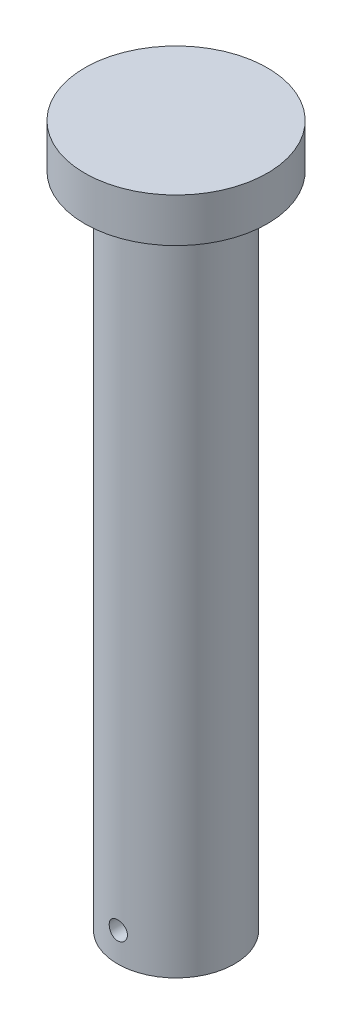
ISO-10303-21;
HEADER;
FILE_DESCRIPTION(('STEP AP214'),'2;1');
FILE_NAME('part.step','',(''),(''),'','','');
FILE_SCHEMA(('AUTOMOTIVE_DESIGN { 1 0 10303 214 1 1 1 1 }'));
ENDSEC;
DATA;
#1=APPLICATION_CONTEXT('core data for automotive mechanical design processes');
#2=APPLICATION_PROTOCOL_DEFINITION('international standard','automotive_design',2000,#1);
#3=PRODUCT_CONTEXT('',#1,'mechanical');
#4=PRODUCT('Part','Part','',(#3));
#5=PRODUCT_RELATED_PRODUCT_CATEGORY('part','',(#4));
#6=PRODUCT_DEFINITION_FORMATION('','',#4);
#7=PRODUCT_DEFINITION_CONTEXT('part definition',#1,'design');
#8=PRODUCT_DEFINITION('design','',#6,#7);
#9=PRODUCT_DEFINITION_SHAPE('','',#8);
#10=(LENGTH_UNIT() NAMED_UNIT(*) SI_UNIT(.MILLI.,.METRE.));
#11=(NAMED_UNIT(*) PLANE_ANGLE_UNIT() SI_UNIT($,.RADIAN.));
#12=(NAMED_UNIT(*) SI_UNIT($,.STERADIAN.) SOLID_ANGLE_UNIT());
#13=UNCERTAINTY_MEASURE_WITH_UNIT(LENGTH_MEASURE(1.E-05),#10,'distance_accuracy_value','');
#14=(GEOMETRIC_REPRESENTATION_CONTEXT(3) GLOBAL_UNCERTAINTY_ASSIGNED_CONTEXT((#13)) GLOBAL_UNIT_ASSIGNED_CONTEXT((#10,
#11,#12)) REPRESENTATION_CONTEXT('',''));
#15=CARTESIAN_POINT('',(0.,0.,0.));
#16=DIRECTION('',(0.,0.,1.));
#17=DIRECTION('',(1.,0.,0.));
#18=AXIS2_PLACEMENT_3D('',#15,#16,#17);
#19=CARTESIAN_POINT('',(0.,12.,0.));
#20=DIRECTION('',(0.,-1.,0.));
#21=DIRECTION('',(0.,0.,-1.));
#22=AXIS2_PLACEMENT_3D('',#19,#20,#21);
#23=CYLINDRICAL_SURFACE('',#22,25.);
#24=CARTESIAN_POINT('',(0.,12.,0.));
#25=DIRECTION('',(0.,1.,0.));
#26=DIRECTION('',(0.,0.,1.));
#27=AXIS2_PLACEMENT_3D('',#24,#25,#26);
#28=CIRCLE('',#27,25.);
#29=CARTESIAN_POINT('',(0.,12.,25.));
#30=VERTEX_POINT('',#29);
#31=EDGE_CURVE('E51',#30,#30,#28,.T.);
#32=ORIENTED_EDGE('',*,*,#31,.F.);
#33=EDGE_LOOP('',(#32));
#34=FACE_BOUND('',#33,.T.);
#35=CARTESIAN_POINT('',(0.,0.,0.));
#36=DIRECTION('',(0.,1.,0.));
#37=DIRECTION('',(0.,0.,1.));
#38=AXIS2_PLACEMENT_3D('',#35,#36,#37);
#39=CIRCLE('',#38,25.);
#40=CARTESIAN_POINT('',(0.,0.,25.));
#41=VERTEX_POINT('',#40);
#42=EDGE_CURVE('E57',#41,#41,#39,.T.);
#43=ORIENTED_EDGE('',*,*,#42,.T.);
#44=EDGE_LOOP('',(#43));
#45=FACE_BOUND('',#44,.T.);
#46=ADVANCED_FACE('F39',(#34,#45),#23,.T.);
#47=CARTESIAN_POINT('',(0.,12.,0.));
#48=DIRECTION('',(0.,1.,0.));
#49=DIRECTION('',(0.,0.,1.));
#50=AXIS2_PLACEMENT_3D('',#47,#48,#49);
#51=PLANE('',#50);
#52=ORIENTED_EDGE('',*,*,#31,.T.);
#53=EDGE_LOOP('',(#52));
#54=FACE_BOUND('',#53,.T.);
#55=ADVANCED_FACE('F87',(#54),#51,.T.);
#56=CARTESIAN_POINT('',(0.,0.,0.));
#57=DIRECTION('',(0.,1.,0.));
#58=DIRECTION('',(0.,0.,1.));
#59=AXIS2_PLACEMENT_3D('',#56,#57,#58);
#60=PLANE('',#59);
#61=CARTESIAN_POINT('',(0.,0.,0.));
#62=DIRECTION('',(0.,-1.,0.));
#63=DIRECTION('',(0.,0.,-1.));
#64=AXIS2_PLACEMENT_3D('',#61,#62,#63);
#65=CIRCLE('',#64,16.);
#66=CARTESIAN_POINT('',(0.,0.,-16.));
#67=VERTEX_POINT('',#66);
#68=EDGE_CURVE('E10',#67,#67,#65,.T.);
#69=ORIENTED_EDGE('',*,*,#68,.F.);
#70=EDGE_LOOP('',(#69));
#71=FACE_BOUND('',#70,.T.);
#72=ORIENTED_EDGE('',*,*,#42,.F.);
#73=EDGE_LOOP('',(#72));
#74=FACE_BOUND('',#73,.T.);
#75=ADVANCED_FACE('F82',(#71,#74),#60,.F.);
#76=CARTESIAN_POINT('',(0.,-180.,0.));
#77=DIRECTION('',(0.,1.,0.));
#78=DIRECTION('',(0.,0.,1.));
#79=AXIS2_PLACEMENT_3D('',#76,#77,#78);
#80=CYLINDRICAL_SURFACE('',#79,16.);
#81=CARTESIAN_POINT('',(0.,-174.5,16.));
#82=CARTESIAN_POINT('',(-0.139515097271032,-174.499994301728,15.9999977019448));
#83=CARTESIAN_POINT('',(-0.279109404865702,-174.488281886226,15.9981561248574));
#84=CARTESIAN_POINT('',(-0.554391314978101,-174.441756308723,15.9909869809759));
#85=CARTESIAN_POINT('',(-0.690075061323318,-174.406921107496,15.9856560884472));
#86=CARTESIAN_POINT('',(-0.953512538047406,-174.315220337193,15.9721069716578));
#87=CARTESIAN_POINT('',(-1.08127235228991,-174.258371918638,15.9638909956317));
#88=CARTESIAN_POINT('',(-1.3254212510446,-174.124301454858,15.9454779403815));
#89=CARTESIAN_POINT('',(-1.44181181036831,-174.047082056964,15.9352811186255));
#90=CARTESIAN_POINT('',(-1.66091991165162,-173.873766951646,15.9139426841436));
#91=CARTESIAN_POINT('',(-1.76352747914264,-173.77753300511,15.9027945139234));
#92=CARTESIAN_POINT('',(-1.95120768822823,-173.569218051731,15.8808607613029));
#93=CARTESIAN_POINT('',(-2.03627928654192,-173.4571361027,15.8700752005075));
#94=CARTESIAN_POINT('',(-2.18690544328884,-173.219561728656,15.8500242812744));
#95=CARTESIAN_POINT('',(-2.25235273557992,-173.094000517638,15.840767397861));
#96=CARTESIAN_POINT('',(-2.36118681597066,-172.833498589142,15.8249120174236));
#97=CARTESIAN_POINT('',(-2.40457491010064,-172.698558427489,15.8183133630222));
#98=CARTESIAN_POINT('',(-2.46771559322167,-172.424289098856,15.8085863451104));
#99=CARTESIAN_POINT('',(-2.48765705487496,-172.285004414181,15.8054302653236));
#100=CARTESIAN_POINT('',(-2.50392369757622,-172.005032811107,15.8028617107177));
#101=CARTESIAN_POINT('',(-2.50025034860466,-171.864345980534,15.8034490028802));
#102=CARTESIAN_POINT('',(-2.4695458080889,-171.586902968147,15.8082755045521));
#103=CARTESIAN_POINT('',(-2.44272562959694,-171.450122776647,15.8124817218495));
#104=CARTESIAN_POINT('',(-2.36681937833752,-171.183027993641,15.8240205634547));
#105=CARTESIAN_POINT('',(-2.31773262684132,-171.052713599359,15.8313532830641));
#106=CARTESIAN_POINT('',(-2.19846916949384,-170.801611287323,15.8483550685462));
#107=CARTESIAN_POINT('',(-2.12820372315549,-170.680866208227,15.8580339308724));
#108=CARTESIAN_POINT('',(-1.96864058146637,-170.452800464314,15.878630461501));
#109=CARTESIAN_POINT('',(-1.87934153253016,-170.345480755113,15.8895482178821));
#110=CARTESIAN_POINT('',(-1.68309088822332,-170.146089753367,15.911537862489));
#111=CARTESIAN_POINT('',(-1.57595800560537,-170.054196841731,15.9226101363559));
#112=CARTESIAN_POINT('',(-1.34769694737934,-169.88966685436,15.9435512534783));
#113=CARTESIAN_POINT('',(-1.22656870068131,-169.817029876443,15.9534200906202));
#114=CARTESIAN_POINT('',(-0.97359592705649,-169.693061926578,15.9708539902704));
#115=CARTESIAN_POINT('',(-0.841744186240456,-169.641745441467,15.9784174854193));
#116=CARTESIAN_POINT('',(-0.571149534696756,-169.562034032553,15.9903756000068));
#117=CARTESIAN_POINT('',(-0.4324071306872,-169.533637425934,15.9947704520898));
#118=CARTESIAN_POINT('',(-0.153508336763736,-169.50081072355,15.9998651172728));
#119=CARTESIAN_POINT('',(-0.0133814615086998,-169.496135521024,16.0006027179286));
#120=CARTESIAN_POINT('',(0.265654546411646,-169.510232705336,15.9984028649127));
#121=CARTESIAN_POINT('',(0.404563719925158,-169.529004302589,15.9954655349964));
#122=CARTESIAN_POINT('',(0.676473446265712,-169.58925838768,15.9862692369322));
#123=CARTESIAN_POINT('',(0.809501262056055,-169.630620758268,15.9800278421539));
#124=CARTESIAN_POINT('',(1.06673406785664,-169.734755094399,15.9649207568356));
#125=CARTESIAN_POINT('',(1.19093861303941,-169.797528138443,15.9560549341007));
#126=CARTESIAN_POINT('',(1.42807220225041,-169.943271991127,15.9365897274094));
#127=CARTESIAN_POINT('',(1.54090512378373,-170.02639742009,15.9259772866342));
#128=CARTESIAN_POINT('',(1.75110696507807,-170.210272085908,15.9042388046444));
#129=CARTESIAN_POINT('',(1.84847490447018,-170.311022439205,15.8931127309268));
#130=CARTESIAN_POINT('',(2.02588080776692,-170.528381197217,15.8714802753665));
#131=CARTESIAN_POINT('',(2.10575398584129,-170.645124847122,15.860980411908));
#132=CARTESIAN_POINT('',(2.24475567726643,-170.890516073661,15.8419069280583));
#133=CARTESIAN_POINT('',(2.30388478778106,-171.019163307489,15.83333325222));
#134=CARTESIAN_POINT('',(2.39946771944995,-171.284229640714,15.8191307135236));
#135=CARTESIAN_POINT('',(2.43600654947913,-171.420617468766,15.8134908234896));
#136=CARTESIAN_POINT('',(2.48564122040535,-171.697689143664,15.8057657028079));
#137=CARTESIAN_POINT('',(2.49873883084997,-171.838372665419,15.8036802038444));
#138=CARTESIAN_POINT('',(2.50107452690756,-172.118398715907,15.8033105804488));
#139=CARTESIAN_POINT('',(2.49057180548425,-172.257739096933,15.804985160429));
#140=CARTESIAN_POINT('',(2.44656223255901,-172.532645297144,15.8118569894183));
#141=CARTESIAN_POINT('',(2.41305543086961,-172.668211124502,15.8170542307995));
#142=CARTESIAN_POINT('',(2.32408329891852,-172.93163782664,15.8303708885491));
#143=CARTESIAN_POINT('',(2.26863761738581,-173.059505478258,15.8384876895341));
#144=CARTESIAN_POINT('',(2.13738768546418,-173.304165613676,15.856731840474));
#145=CARTESIAN_POINT('',(2.06158262820886,-173.420957658288,15.8668592701083));
#146=CARTESIAN_POINT('',(1.89083008139079,-173.641465544127,15.8881156809226));
#147=CARTESIAN_POINT('',(1.79569107094767,-173.745032196614,15.8992540116029));
#148=CARTESIAN_POINT('',(1.58937594638203,-173.934821236387,15.9212004364073));
#149=CARTESIAN_POINT('',(1.47819612078432,-174.021039598592,15.9320084534012));
#150=CARTESIAN_POINT('',(1.24216685884341,-174.174151223032,15.952151024567));
#151=CARTESIAN_POINT('',(1.11723937214237,-174.24092537276,15.9614763443027));
#152=CARTESIAN_POINT('',(0.857851882357781,-174.352440996193,15.9775125983888));
#153=CARTESIAN_POINT('',(0.723401776581768,-174.397204972558,15.9842262014212));
#154=CARTESIAN_POINT('',(0.490314239911604,-174.453433021091,15.9927744586488));
#155=CARTESIAN_POINT('',(0.393105575651631,-174.470868490629,15.9954699162612));
#156=CARTESIAN_POINT('',(0.197277797850584,-174.494153913379,15.9990834869762));
#157=CARTESIAN_POINT('',(0.0986587041691198,-174.500004029557,16.0000016250796));
#158=CARTESIAN_POINT('',(0.,-174.5,16.));
#159=B_SPLINE_CURVE_WITH_KNOTS('',3,(#81,#82,#83,#84,#85,#86,#87,#88,#89,#90,#91,#92,#93,#94,
#95,#96,#97,#98,#99,#100,#101,#102,#103,#104,#105,#106,#107,#108,#109,#110,#111,#112,#113,#114,
#115,#116,#117,#118,#119,#120,#121,#122,#123,#124,#125,#126,#127,#128,#129,#130,#131,#132,#133,
#134,#135,#136,#137,#138,#139,#140,#141,#142,#143,#144,#145,#146,#147,#148,#149,#150,#151,#152,
#153,#154,#155,#156,#157,#158),.UNSPECIFIED.,.T.,.F.,(4,2,2,2,2,2,2,2,2,2,2,2,2,2,2,2,2,2,2,2,2,
2,2,2,2,2,2,2,2,2,2,2,2,2,2,2,2,2,4),(0.,0.418184740477489,0.836768642528017,1.25502707944104,
1.6732311879203,2.09459568152198,2.51598523645421,2.9396377860576,3.36326525009242,
3.78345631134993,4.20362121670544,4.61999576022579,5.0363829965105,5.45453977402348,
5.87272629892068,6.29545732334371,6.71819049513828,7.14121043754565,7.56419931829866,
7.98280854005915,8.40140366528357,8.81779444756568,9.23420620742031,9.65388541469672,
10.0735912160142,10.497094802496,10.9205861964898,11.3424741039513,11.764330162293,
12.1815758159869,12.598820566189,13.0156924696662,13.4325808967135,13.8538201231554,
14.275156971423,14.6990230419984,15.1224548565628,15.4181801635154,15.7139013105871),.UNSPECIFIED.);
#160=CARTESIAN_POINT('',(0.,-174.5,16.));
#161=VERTEX_POINT('',#160);
#162=EDGE_CURVE('E45',#161,#161,#159,.T.);
#163=ORIENTED_EDGE('',*,*,#162,.T.);
#164=EDGE_LOOP('',(#163));
#165=FACE_BOUND('',#164,.T.);
#166=CARTESIAN_POINT('',(2.5,-172.,-15.8034806292791));
#167=CARTESIAN_POINT('',(2.49999429179104,-171.860496621659,-15.8034830346332));
#168=CARTESIAN_POINT('',(2.48828377742084,-171.720914002315,-15.8053478026579));
#169=CARTESIAN_POINT('',(2.44176643645043,-171.445656370997,-15.8125997089633));
#170=CARTESIAN_POINT('',(2.40693752801736,-171.309985224521,-15.8179902148259));
#171=CARTESIAN_POINT('',(2.31525516047132,-171.046574410356,-15.8316684916183));
#172=CARTESIAN_POINT('',(2.25841914921921,-170.918828552129,-15.8399539668268));
#173=CARTESIAN_POINT('',(2.12437791816389,-170.674703109158,-15.8584858981599));
#174=CARTESIAN_POINT('',(2.04717531605121,-170.55832206634,-15.8687321022282));
#175=CARTESIAN_POINT('',(1.8738773011091,-170.339203514849,-15.8901303851737));
#176=CARTESIAN_POINT('',(1.77763988617498,-170.2365789256,-15.9012888784461));
#177=CARTESIAN_POINT('',(1.5693108098767,-170.04886577957,-15.9231973082666));
#178=CARTESIAN_POINT('',(1.45721825316847,-169.963778213776,-15.9339472216984));
#179=CARTESIAN_POINT('',(1.2196342918576,-169.813135122959,-15.9538946715316));
#180=CARTESIAN_POINT('',(1.09407592635728,-169.747683996026,-15.9630838016344));
#181=CARTESIAN_POINT('',(0.833580171794749,-169.638842045275,-15.978803149105));
#182=CARTESIAN_POINT('',(0.698643320136801,-169.595449958617,-15.9853335186778));
#183=CARTESIAN_POINT('',(0.424385325448801,-169.532301281044,-15.9949542857973));
#184=CARTESIAN_POINT('',(0.285108760160741,-169.512355350932,-15.9980722260505));
#185=CARTESIAN_POINT('',(0.0051531435506613,-169.496076956697,-16.0006113098095));
#186=CARTESIAN_POINT('',(-0.135525822989196,-169.499743073648,-16.0000326754547));
#187=CARTESIAN_POINT('',(-0.413000089722162,-169.530435926278,-15.9952657389868));
#188=CARTESIAN_POINT('',(-0.549818542575187,-169.55725893884,-15.9911089169598));
#189=CARTESIAN_POINT('',(-0.816988375343502,-169.633184028623,-15.9796877395528));
#190=CARTESIAN_POINT('',(-0.947339577352183,-169.682286718354,-15.9724232987387));
#191=CARTESIAN_POINT('',(-1.19848742679248,-169.80158365586,-15.9555491842028));
#192=CARTESIAN_POINT('',(-1.31924299071838,-169.871863005428,-15.9459300777042));
#193=CARTESIAN_POINT('',(-1.54732385653215,-170.031456080629,-15.9254174702046));
#194=CARTESIAN_POINT('',(-1.65464819959325,-170.120771163955,-15.9145238783282));
#195=CARTESIAN_POINT('',(-1.85402198520022,-170.317033487073,-15.8925387825556));
#196=CARTESIAN_POINT('',(-1.94589625613073,-170.424158666395,-15.8814464071021));
#197=CARTESIAN_POINT('',(-2.11039226047484,-170.652397564682,-15.8604269384475));
#198=CARTESIAN_POINT('',(-2.18301385538335,-170.773511384274,-15.8504998536298));
#199=CARTESIAN_POINT('',(-2.30697060635686,-171.026479628106,-15.8329349281613));
#200=CARTESIAN_POINT('',(-2.35828663884161,-171.158343575073,-15.8252991458489));
#201=CARTESIAN_POINT('',(-2.43799343127668,-171.428964848705,-15.8132168990948));
#202=CARTESIAN_POINT('',(-2.46638595195258,-171.56772164507,-15.8087701897074));
#203=CARTESIAN_POINT('',(-2.49919719237856,-171.846628103275,-15.8036163696886));
#204=CARTESIAN_POINT('',(-2.50386473411271,-171.986747800195,-15.80287044806));
#205=CARTESIAN_POINT('',(-2.48975479033184,-172.265767635298,-15.8050994977182));
#206=CARTESIAN_POINT('',(-2.47097809654328,-172.404667814506,-15.8080743433524));
#207=CARTESIAN_POINT('',(-2.41072412555895,-172.676527807466,-15.8173740105186));
#208=CARTESIAN_POINT('',(-2.36937178781978,-172.80951599864,-15.8236803883335));
#209=CARTESIAN_POINT('',(-2.26527072241931,-173.066673971104,-15.8389172439685));
#210=CARTESIAN_POINT('',(-2.20252085602949,-173.190843282649,-15.8478478614411));
#211=CARTESIAN_POINT('',(-2.05681199170293,-173.427951281649,-15.8674179220711));
#212=CARTESIAN_POINT('',(-1.9736925109347,-173.5407902289,-15.8780706945976));
#213=CARTESIAN_POINT('',(-1.78982593995281,-173.751006980848,-15.8998450469621));
#214=CARTESIAN_POINT('',(-1.6890777652142,-173.848383833607,-15.9109666556111));
#215=CARTESIAN_POINT('',(-1.47171546765808,-174.025811270635,-15.9325473887455));
#216=CARTESIAN_POINT('',(-1.35496564158983,-174.10569657643,-15.9429995842164));
#217=CARTESIAN_POINT('',(-1.10955861029336,-174.24471951999,-15.9619548934084));
#218=CARTESIAN_POINT('',(-0.980901753162473,-174.303857764046,-15.9704580640831));
#219=CARTESIAN_POINT('',(-0.715839663778304,-174.399446275284,-15.9845269767683));
#220=CARTESIAN_POINT('',(-0.579467147617065,-174.435985497439,-15.9901042225572));
#221=CARTESIAN_POINT('',(-0.302427949770724,-174.485626132673,-15.9977412978946));
#222=CARTESIAN_POINT('',(-0.161761577654413,-174.498729231356,-15.9998013804089));
#223=CARTESIAN_POINT('',(0.118272165188282,-174.501081852655,-16.0001691012796));
#224=CARTESIAN_POINT('',(0.257637428859796,-174.490583744643,-15.9985164403994));
#225=CARTESIAN_POINT('',(0.53259459546489,-174.44657468382,-15.9917247801431));
#226=CARTESIAN_POINT('',(0.66818651358165,-174.413063823622,-15.9865857947973));
#227=CARTESIAN_POINT('',(0.931668850429406,-174.324072740288,-15.9733964142131));
#228=CARTESIAN_POINT('',(1.05956579651625,-174.268611448419,-15.965348528289));
#229=CARTESIAN_POINT('',(1.30427807253219,-174.137321161478,-15.947223323121));
#230=CARTESIAN_POINT('',(1.42109298145458,-174.061491393026,-15.9371459268214));
#231=CARTESIAN_POINT('',(1.64160219185803,-173.890710556792,-15.9159528222148));
#232=CARTESIAN_POINT('',(1.74515169482399,-173.795573685696,-15.9048276353277));
#233=CARTESIAN_POINT('',(1.93490712736947,-173.589270042665,-15.8828612878644));
#234=CARTESIAN_POINT('',(2.02110898563013,-173.478099518275,-15.8720201944801));
#235=CARTESIAN_POINT('',(2.17420151541623,-173.242078895725,-15.8517779742959));
#236=CARTESIAN_POINT('',(2.24097044145098,-173.11714904139,-15.842386091806));
#237=CARTESIAN_POINT('',(2.35247565604315,-172.85775678237,-15.8262143333515));
#238=CARTESIAN_POINT('',(2.3972345005847,-172.723304298883,-15.8194317848938));
#239=CARTESIAN_POINT('',(2.45344906957714,-172.490230260304,-15.8107909670081));
#240=CARTESIAN_POINT('',(2.47087849275467,-172.393038400015,-15.8080643798014));
#241=CARTESIAN_POINT('',(2.49415589078729,-172.197244218954,-15.804408373768));
#242=CARTESIAN_POINT('',(2.50000403623692,-172.098641918978,-15.803478928469));
#243=CARTESIAN_POINT('',(2.5,-172.,-15.8034806292791));
#244=B_SPLINE_CURVE_WITH_KNOTS('',3,(#166,#167,#168,#169,#170,#171,#172,#173,#174,#175,#176,
#177,#178,#179,#180,#181,#182,#183,#184,#185,#186,#187,#188,#189,#190,#191,#192,#193,#194,#195,
#196,#197,#198,#199,#200,#201,#202,#203,#204,#205,#206,#207,#208,#209,#210,#211,#212,#213,#214,
#215,#216,#217,#218,#219,#220,#221,#222,#223,#224,#225,#226,#227,#228,#229,#230,#231,#232,#233,
#234,#235,#236,#237,#238,#239,#240,#241,#242,#243),.UNSPECIFIED.,.T.,.F.,(4,2,2,2,2,2,2,2,2,2,2,
2,2,2,2,2,2,2,2,2,2,2,2,2,2,2,2,2,2,2,2,2,2,2,2,2,2,2,4),(0.,0.41814952790225,0.836699032574088,
1.25491737645053,1.67308199345223,2.09449258051087,2.51592697424483,2.93956378022296,
3.36317633102574,3.78334397517518,4.20348637030327,4.61996979150786,5.03646466334576,
5.45465612930834,5.87287743207565,6.29556043395284,6.71824647655855,7.14131110038651,
7.56434322607052,7.98292940034461,8.40150143908465,8.81778013452042,9.23408098683357,
9.65377352836982,10.0734918986585,10.4970197199929,10.9205351635679,11.3423727623224,
11.7641800198745,12.18149834073,12.5988149821383,13.0157724881518,13.432745828047,
13.8539404040181,14.275233715164,14.6991122166339,15.1225554163993,15.4182305458031,
15.7139013198206),.UNSPECIFIED.);
#245=CARTESIAN_POINT('',(2.5,-172.,-15.8034806292791));
#246=VERTEX_POINT('',#245);
#247=EDGE_CURVE('E64',#246,#246,#244,.T.);
#248=ORIENTED_EDGE('',*,*,#247,.T.);
#249=EDGE_LOOP('',(#248));
#250=FACE_BOUND('',#249,.T.);
#251=CARTESIAN_POINT('',(0.,-180.,0.));
#252=DIRECTION('',(0.,-1.,0.));
#253=DIRECTION('',(0.,0.,-1.));
#254=AXIS2_PLACEMENT_3D('',#251,#252,#253);
#255=CIRCLE('',#254,16.);
#256=CARTESIAN_POINT('',(0.,-180.,-16.));
#257=VERTEX_POINT('',#256);
#258=EDGE_CURVE('E56',#257,#257,#255,.T.);
#259=ORIENTED_EDGE('',*,*,#258,.F.);
#260=EDGE_LOOP('',(#259));
#261=FACE_BOUND('',#260,.T.);
#262=ORIENTED_EDGE('',*,*,#68,.T.);
#263=EDGE_LOOP('',(#262));
#264=FACE_BOUND('',#263,.T.);
#265=ADVANCED_FACE('F69',(#165,#250,#261,#264),#80,.T.);
#266=CARTESIAN_POINT('',(0.,-180.,0.));
#267=DIRECTION('',(0.,-1.,0.));
#268=DIRECTION('',(0.,0.,-1.));
#269=AXIS2_PLACEMENT_3D('',#266,#267,#268);
#270=PLANE('',#269);
#271=ORIENTED_EDGE('',*,*,#258,.T.);
#272=EDGE_LOOP('',(#271));
#273=FACE_BOUND('',#272,.T.);
#274=ADVANCED_FACE('F74',(#273),#270,.T.);
#275=CARTESIAN_POINT('',(0.,-172.,-90.));
#276=DIRECTION('',(0.,0.,1.));
#277=DIRECTION('',(1.,0.,0.));
#278=AXIS2_PLACEMENT_3D('',#275,#276,#277);
#279=CYLINDRICAL_SURFACE('',#278,2.5);
#280=ORIENTED_EDGE('',*,*,#247,.F.);
#281=EDGE_LOOP('',(#280));
#282=FACE_BOUND('',#281,.T.);
#283=ORIENTED_EDGE('',*,*,#162,.F.);
#284=EDGE_LOOP('',(#283));
#285=FACE_BOUND('',#284,.T.);
#286=ADVANCED_FACE('F72',(#282,#285),#279,.F.);
#287=CLOSED_SHELL('',(#46,#55,#75,#265,#274,#286));
#288=MANIFOLD_SOLID_BREP('B2',#287);
#289=ADVANCED_BREP_SHAPE_REPRESENTATION('',(#18,#288),#14);
#290=SHAPE_DEFINITION_REPRESENTATION(#9,#289);
ENDSEC;
END-ISO-10303-21;
